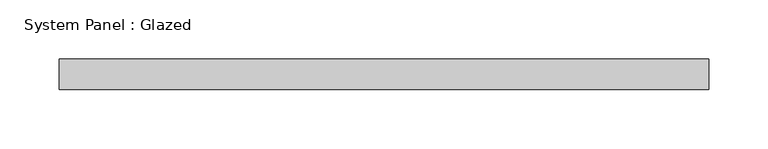
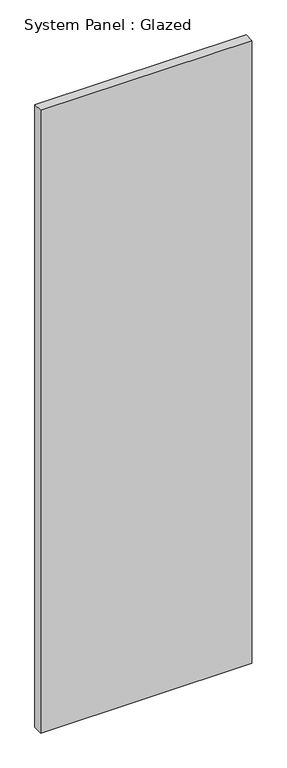
"""IFC4 building model written with IfcOpenShell, lengths in millimetres: plate geometry, System Panel : Glazed."""

from ifc_helpers import new_model, si_unit, origin, origin_with_axes, place, context, project, spatial, polyline, outline, extrude, source, transform, mapped, element, save


def system_panel_glazed_2a291ae9(model_context):
    return source(origin(), model_context, "Body", "SweptSolid", [
        extrude(outline(polyline([(273.05, 19.05), (-273.05, 19.05), (-273.05, 44.45), (273.05, 44.45), (273.05, 19.05)])), origin_with_axes(), (0.0, 0.0, 1.0), 1701.8),
    ])


if __name__ == "__main__":
    model = new_model("IFC4")
    model_context = context("Model", 3, world=origin())
    ifc_project = project(units=[si_unit("LENGTHUNIT", "METRE", prefix="MILLI")], contexts=[model_context])
    site = spatial("IfcSite", under=ifc_project)
    building = spatial("IfcBuilding", under=site)
    placement = place(None, origin())
    system_panel_glazed_shape = system_panel_glazed_2a291ae9(model_context)
    element("IfcPlate", 1, ObjectType="System Panel : Glazed", at=placement, inside=building, context=model_context, shape_type="MappedRepresentation", body=[
        mapped(system_panel_glazed_shape, transform((0.0, 0.0, 0.0), x_axis=(1.0, 0.0, 0.0), y_axis=(0.0, 1.0, 0.0), z_axis=(0.0, 0.0, 1.0))),
    ])
    save(model, "model.ifc")

# Revit data of these elements
# Type "System Panel : Glazed"
#   Construction Type Id = "GSP4R"
#   Analytic Construction = "1/8 in Pilkington single glazing"
#   Visual Light Transmittance = 0.9
#   Solar Heat Gain Coefficient = 0.86
#   Heat Transfer Coefficient (U) = 1.18115 BTU/(h·ft²·°F)
#   Define Thermal Properties by = 1
# Element 1 (IfcPlate, "System Panel : Glazed")
#   Materials on its faces: "Glass"
# Materials
#   "Glass": class "Glass", colour RGB 0 128 192, transparency 0.75, Description = "Soda Lime Glass", Cost = 0
